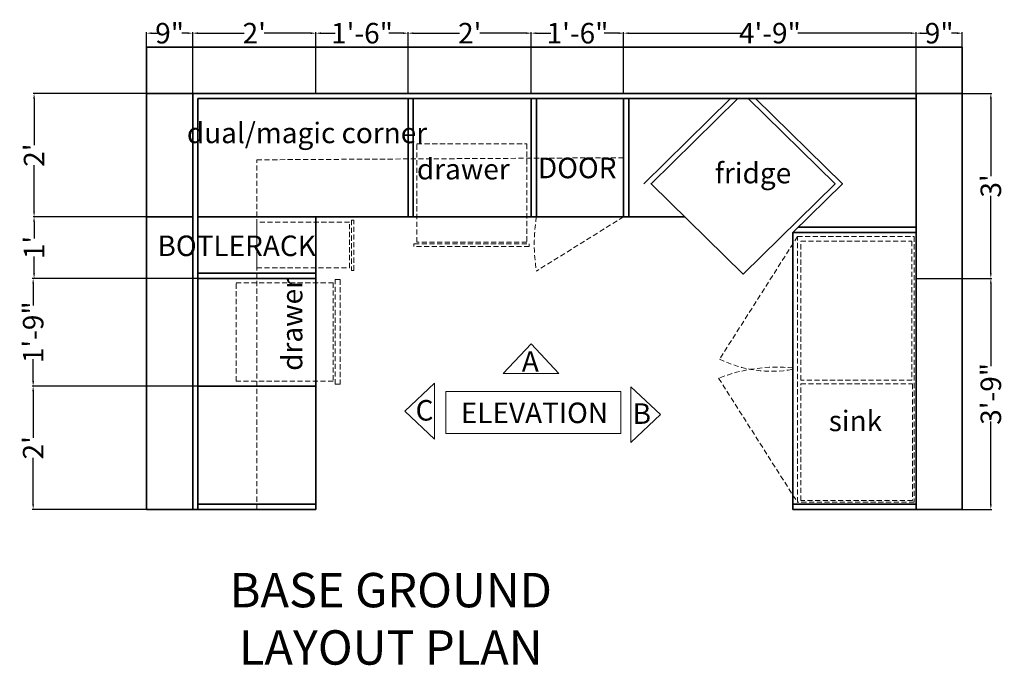
# Model space of a CAD drawing. Units: inches. Extents: x 560 to 756, y 301 to 635.
# Tile 2 of 2: x 564 to 756, y 509 to 635. Entities that reach past the tile are written whole.
import ezdxf

# ---------------------------------------------------------------- set-up
doc = ezdxf.new("R2010")
doc.units = ezdxf.units.IN
doc.header["$LTSCALE"] = 2
doc.header["$MEASUREMENT"] = 0
doc.linetypes.add('DASHED', pattern=[0.75, 0.5, -0.25])
for name, color, linetype, lineweight in [('A-ANNO-DIMS', 2, 'Continuous', 18), ('A-ANNO-SYMB', 7, 'Continuous', 18), ('A-ANNO-TEXT', 3, 'Continuous', 18), ('A-FURN', 7, 'Continuous', 35), ('A-FURN-OPEN', 8, 'DASHED', 18)]:
    doc.layers.add(name, color=color, linetype=linetype, lineweight=lineweight)
doc.styles.get("Standard").update_dxf_attribs({"font": 'arial.ttf'})
doc.dimstyles.get("Standard").update_dxf_attribs({"dimtxt": 4, "dimasz": 1, "dimexe": 0.18, "dimexo": 0.0625, "dimgap": 0.09, "dimtad": 0, "dimdec": 0, "dimzin": 0, "dimdsep": 46, "dimlunit": 4, "dimtxsty": 'Standard', "dimcen": 0.09, "dimadec": 0, "dimazin": 0, "dimtfac": 1, "dimtdec": 0, "dimtofl": 0, "dimtmove": 0, "dimatfit": 3, "dimfxl": 1, "dimtolj": 1, "dimtzin": 0, "dimarcsym": 0})

# ---------------------------------------------------------------- blocks, each defined once
blk = doc.blocks.new('*D1')
at = {"layer": 'A-ANNO-DIMS', "color": 0, "lineweight": -2, "transparency": 16777216}
for p, q in [((589.13, 620.48), (589.13, 632.34)), ((590.13, 632.16), (591.24, 632.16)), ((597.13, 632.16), (596.02, 632.16)), ((598.13, 620.48), (598.13, 632.34))]:
    blk.add_line(p, q, dxfattribs=at)
at = {"layer": 'A-ANNO-DIMS', "color": 0, "transparency": 16777216}
for points in [[(590.13, 632.33), (590.13, 632), (589.13, 632.16)], [(597.13, 632.33), (597.13, 632), (598.13, 632.16)]]:
    blk.add_solid(points, dxfattribs=at)
at = {"layer": 'Defpoints', "color": 0, "transparency": 16777216}
for p in [(598.13, 632.16), (589.13, 620.41), (598.13, 620.41)]:
    blk.add_point(p, dxfattribs=at)
at = {"layer": 'A-ANNO-DIMS', "color": 0, "transparency": 16777216, "insert": (593.63, 632.16), "char_height": 4, "attachment_point": 5}
blk.add_mtext('\\A1;9"', dxfattribs=at)
blk = doc.blocks.new('*D2')
at = {"layer": 'A-ANNO-DIMS', "color": 0, "lineweight": -2, "transparency": 16777216}
for p, q in [((598.13, 620.48), (598.13, 632.34)), ((599.13, 632.16), (608.16, 632.16)), ((621.13, 632.16), (612.09, 632.16)), ((622.13, 620.48), (622.13, 632.34))]:
    blk.add_line(p, q, dxfattribs=at)
at = {"layer": 'A-ANNO-DIMS', "color": 0, "transparency": 16777216}
for points in [[(599.13, 632.33), (599.13, 632), (598.13, 632.16)], [(621.13, 632.33), (621.13, 632), (622.13, 632.16)]]:
    blk.add_solid(points, dxfattribs=at)
at = {"layer": 'Defpoints', "color": 0, "transparency": 16777216}
for p in [(622.13, 632.16), (598.13, 620.41), (622.13, 620.41)]:
    blk.add_point(p, dxfattribs=at)
at = {"layer": 'A-ANNO-DIMS', "color": 0, "transparency": 16777216, "insert": (610.13, 632.16), "char_height": 4, "attachment_point": 5}
blk.add_mtext("\\A1;2'", dxfattribs=at)
blk = doc.blocks.new('*D3')
at = {"layer": 'A-ANNO-DIMS', "color": 0, "lineweight": -2, "transparency": 16777216}
for p, q in [((622.13, 620.48), (622.13, 632.34)), ((623.13, 632.16), (625.91, 632.16)), ((639.13, 632.16), (636.35, 632.16)), ((640.13, 620.48), (640.13, 632.34))]:
    blk.add_line(p, q, dxfattribs=at)
at = {"layer": 'A-ANNO-DIMS', "color": 0, "transparency": 16777216}
for points in [[(623.13, 632.33), (623.13, 632), (622.13, 632.16)], [(639.13, 632.33), (639.13, 632), (640.13, 632.16)]]:
    blk.add_solid(points, dxfattribs=at)
at = {"layer": 'Defpoints', "color": 0, "transparency": 16777216}
for p in [(640.13, 632.16), (622.13, 620.41), (640.13, 620.41)]:
    blk.add_point(p, dxfattribs=at)
at = {"layer": 'A-ANNO-DIMS', "color": 0, "transparency": 16777216, "insert": (631.13, 632.16), "char_height": 4, "attachment_point": 5}
blk.add_mtext('\\A1;1\'-6"', dxfattribs=at)
blk = doc.blocks.new('*D4')
at = {"layer": 'A-ANNO-DIMS', "color": 0, "lineweight": -2, "transparency": 16777216}
for p, q in [((640.13, 620.48), (640.13, 632.34)), ((641.13, 632.16), (650.16, 632.16)), ((663.13, 632.16), (654.09, 632.16)), ((664.13, 620.48), (664.13, 632.34))]:
    blk.add_line(p, q, dxfattribs=at)
at = {"layer": 'A-ANNO-DIMS', "color": 0, "transparency": 16777216}
for points in [[(641.13, 632.33), (641.13, 632), (640.13, 632.16)], [(663.13, 632.33), (663.13, 632), (664.13, 632.16)]]:
    blk.add_solid(points, dxfattribs=at)
at = {"layer": 'Defpoints', "color": 0, "transparency": 16777216}
for p in [(664.13, 632.16), (640.13, 620.41), (664.13, 620.41)]:
    blk.add_point(p, dxfattribs=at)
at = {"layer": 'A-ANNO-DIMS', "color": 0, "transparency": 16777216, "insert": (652.13, 632.16), "char_height": 4, "attachment_point": 5}
blk.add_mtext("\\A1;2'", dxfattribs=at)
blk = doc.blocks.new('*D5')
at = {"layer": 'A-ANNO-DIMS', "color": 0, "lineweight": -2, "transparency": 16777216}
for p, q in [((664.13, 620.48), (664.13, 632.34)), ((665.13, 632.16), (667.91, 632.16)), ((681.13, 632.16), (678.35, 632.16)), ((682.13, 620.48), (682.13, 632.34))]:
    blk.add_line(p, q, dxfattribs=at)
at = {"layer": 'A-ANNO-DIMS', "color": 0, "transparency": 16777216}
for points in [[(665.13, 632.33), (665.13, 632), (664.13, 632.16)], [(681.13, 632.33), (681.13, 632), (682.13, 632.16)]]:
    blk.add_solid(points, dxfattribs=at)
at = {"layer": 'Defpoints', "color": 0, "transparency": 16777216}
for p in [(682.13, 632.16), (664.13, 620.41), (682.13, 620.41)]:
    blk.add_point(p, dxfattribs=at)
at = {"layer": 'A-ANNO-DIMS', "color": 0, "transparency": 16777216, "insert": (673.13, 632.16), "char_height": 4, "attachment_point": 5}
blk.add_mtext('\\A1;1\'-6"', dxfattribs=at)
blk = doc.blocks.new('*D6')
at = {"layer": 'A-ANNO-DIMS', "color": 0, "lineweight": -2, "transparency": 16777216}
for p, q in [((682.13, 620.48), (682.13, 632.34)), ((683.13, 632.16), (705.14, 632.16)), ((738.13, 632.16), (716.11, 632.16)), ((739.13, 620.48), (739.13, 632.34))]:
    blk.add_line(p, q, dxfattribs=at)
at = {"layer": 'A-ANNO-DIMS', "color": 0, "transparency": 16777216}
for points in [[(683.13, 632.33), (683.13, 632), (682.13, 632.16)], [(738.13, 632.33), (738.13, 632), (739.13, 632.16)]]:
    blk.add_solid(points, dxfattribs=at)
at = {"layer": 'Defpoints', "color": 0, "transparency": 16777216}
for p in [(739.13, 632.16), (682.13, 620.41), (739.13, 620.41)]:
    blk.add_point(p, dxfattribs=at)
at = {"layer": 'A-ANNO-DIMS', "color": 0, "transparency": 16777216, "insert": (710.63, 632.16), "char_height": 4, "attachment_point": 5}
blk.add_mtext('\\A1;4\'-9"', dxfattribs=at)
blk = doc.blocks.new('*D7')
at = {"layer": 'A-ANNO-DIMS', "color": 0, "lineweight": -2, "transparency": 16777216}
for p, q in [((739.13, 620.48), (739.13, 632.34)), ((740.13, 632.16), (741.24, 632.16)), ((747.13, 632.16), (746.02, 632.16)), ((748.13, 620.48), (748.13, 632.34))]:
    blk.add_line(p, q, dxfattribs=at)
at = {"layer": 'A-ANNO-DIMS', "color": 0, "transparency": 16777216}
for points in [[(740.13, 632.33), (740.13, 632), (739.13, 632.16)], [(747.13, 632.33), (747.13, 632), (748.13, 632.16)]]:
    blk.add_solid(points, dxfattribs=at)
at = {"layer": 'Defpoints', "color": 0, "transparency": 16777216}
for p in [(739.13, 632.16), (739.13, 620.41), (748.13, 620.41)]:
    blk.add_point(p, dxfattribs=at)
at = {"layer": 'A-ANNO-DIMS', "color": 0, "transparency": 16777216, "insert": (743.63, 632.16), "char_height": 4, "attachment_point": 5}
blk.add_mtext('\\A1;9"', dxfattribs=at)
blk = doc.blocks.new('*D8')
at = {"layer": 'A-ANNO-DIMS', "color": 0, "lineweight": -2, "transparency": 16777216}
for p, q in [((589.06, 620.41), (567.03, 620.41)), ((567.21, 619.41), (567.21, 610.38)), ((567.21, 597.41), (567.21, 606.45)), ((589.06, 596.41), (567.03, 596.41))]:
    blk.add_line(p, q, dxfattribs=at)
at = {"layer": 'A-ANNO-DIMS', "color": 0, "transparency": 16777216}
for points in [[(567.04, 619.41), (567.38, 619.41), (567.21, 620.41)], [(567.04, 597.41), (567.38, 597.41), (567.21, 596.41)]]:
    blk.add_solid(points, dxfattribs=at)
at = {"layer": 'Defpoints', "color": 0, "transparency": 16777216}
for p in [(589.13, 620.41), (567.21, 596.41), (589.13, 596.41)]:
    blk.add_point(p, dxfattribs=at)
at = {"layer": 'A-ANNO-DIMS', "color": 0, "transparency": 16777216, "insert": (567.21, 608.41), "char_height": 4, "attachment_point": 5, "rotation": 90}
blk.add_mtext("\\A1;2'", dxfattribs=at)
blk = doc.blocks.new('*D9')
at = {"layer": 'A-ANNO-DIMS', "color": 0, "lineweight": -2, "transparency": 16777216}
for p, q in [((598.06, 596.41), (567.03, 596.41)), ((567.21, 595.41), (567.21, 592.16)), ((567.21, 585.41), (567.21, 588.67)), ((598.06, 584.41), (567.03, 584.41))]:
    blk.add_line(p, q, dxfattribs=at)
at = {"layer": 'A-ANNO-DIMS', "color": 0, "transparency": 16777216}
for points in [[(567.04, 595.41), (567.38, 595.41), (567.21, 596.41)], [(567.04, 585.41), (567.38, 585.41), (567.21, 584.41)]]:
    blk.add_solid(points, dxfattribs=at)
at = {"layer": 'Defpoints', "color": 0, "transparency": 16777216}
for p in [(598.13, 596.41), (567.21, 584.41), (598.13, 584.41)]:
    blk.add_point(p, dxfattribs=at)
at = {"layer": 'A-ANNO-DIMS', "color": 0, "transparency": 16777216, "insert": (567.21, 590.41), "char_height": 4, "attachment_point": 5, "rotation": 90}
blk.add_mtext("\\A1;1'", dxfattribs=at)
blk = doc.blocks.new('*D10')
at = {"layer": 'A-ANNO-DIMS', "color": 0, "lineweight": -2, "transparency": 16777216}
for p, q in [((739.19, 620.41), (753.88, 620.41)), ((753.7, 619.41), (753.7, 604.34)), ((753.7, 585.41), (753.7, 600.49)), ((739.19, 584.41), (753.88, 584.41))]:
    blk.add_line(p, q, dxfattribs=at)
at = {"layer": 'A-ANNO-DIMS', "color": 0, "transparency": 16777216}
for points in [[(753.53, 619.41), (753.87, 619.41), (753.7, 620.41)], [(753.53, 585.41), (753.87, 585.41), (753.7, 584.41)]]:
    blk.add_solid(points, dxfattribs=at)
at = {"layer": 'Defpoints', "color": 0, "transparency": 16777216}
for p in [(739.13, 620.41), (739.13, 584.41), (753.7, 584.41)]:
    blk.add_point(p, dxfattribs=at)
at = {"layer": 'A-ANNO-DIMS', "color": 0, "transparency": 16777216, "insert": (753.7, 602.41), "char_height": 4, "attachment_point": 5, "rotation": 90}
blk.add_mtext("\\A1;3'", dxfattribs=at)
blk = doc.blocks.new('*D11')
at = {"layer": 'A-ANNO-DIMS', "color": 0, "lineweight": -2, "transparency": 16777216}
for p, q in [((739.19, 584.41), (753.88, 584.41)), ((753.7, 583.41), (753.7, 567.32)), ((753.7, 540.41), (753.7, 556.51)), ((739.19, 539.41), (753.88, 539.41))]:
    blk.add_line(p, q, dxfattribs=at)
at = {"layer": 'A-ANNO-DIMS', "color": 0, "transparency": 16777216}
for points in [[(753.53, 583.41), (753.87, 583.41), (753.7, 584.41)], [(753.53, 540.41), (753.87, 540.41), (753.7, 539.41)]]:
    blk.add_solid(points, dxfattribs=at)
at = {"layer": 'Defpoints', "color": 0, "transparency": 16777216}
for p in [(739.13, 584.41), (739.13, 539.41), (753.7, 539.41)]:
    blk.add_point(p, dxfattribs=at)
at = {"layer": 'A-ANNO-DIMS', "color": 0, "transparency": 16777216, "insert": (753.7, 561.91), "char_height": 4, "attachment_point": 5, "rotation": 90}
blk.add_mtext('\\A1;3\'-9"', dxfattribs=at)
blk = doc.blocks.new('*D12')
at = {"layer": 'A-ANNO-DIMS', "color": 0, "lineweight": -2, "transparency": 16777216}
for p, q in [((599.06, 584.41), (566.85, 584.41)), ((567.03, 583.41), (567.03, 579.13)), ((567.03, 564.41), (567.03, 568.7)), ((599.06, 563.41), (566.85, 563.41))]:
    blk.add_line(p, q, dxfattribs=at)
at = {"layer": 'A-ANNO-DIMS', "color": 0, "transparency": 16777216}
for points in [[(566.86, 583.41), (567.2, 583.41), (567.03, 584.41)], [(566.86, 564.41), (567.2, 564.41), (567.03, 563.41)]]:
    blk.add_solid(points, dxfattribs=at)
at = {"layer": 'Defpoints', "color": 0, "transparency": 16777216}
for p in [(599.13, 584.41), (567.03, 563.41), (599.13, 563.41)]:
    blk.add_point(p, dxfattribs=at)
at = {"layer": 'A-ANNO-DIMS', "color": 0, "transparency": 16777216, "insert": (567.03, 573.91), "char_height": 4, "attachment_point": 5, "rotation": 90}
blk.add_mtext('\\A1;1\'-9"', dxfattribs=at)
blk = doc.blocks.new('*D13')
at = {"layer": 'A-ANNO-DIMS', "color": 0, "lineweight": -2, "transparency": 16777216}
for p, q in [((589.06, 563.41), (566.85, 563.41)), ((567.03, 562.41), (567.03, 553.38)), ((567.03, 540.41), (567.03, 549.45)), ((589.06, 539.41), (566.85, 539.41))]:
    blk.add_line(p, q, dxfattribs=at)
at = {"layer": 'A-ANNO-DIMS', "color": 0, "transparency": 16777216}
for points in [[(566.86, 562.41), (567.2, 562.41), (567.03, 563.41)], [(566.86, 540.41), (567.2, 540.41), (567.03, 539.41)]]:
    blk.add_solid(points, dxfattribs=at)
at = {"layer": 'Defpoints', "color": 0, "transparency": 16777216}
for p in [(589.13, 563.41), (567.03, 539.41), (589.13, 539.41)]:
    blk.add_point(p, dxfattribs=at)
at = {"layer": 'A-ANNO-DIMS', "color": 0, "transparency": 16777216, "insert": (567.03, 551.41), "char_height": 4, "attachment_point": 5, "rotation": 90}
blk.add_mtext("\\A1;2'", dxfattribs=at)

msp = doc.modelspace()

# ---------------------------------------------------------------- linework, layer by layer
at = {"layer": 'A-ANNO-SYMB'}
for points in [[(658.64, 565.87), (669.52, 565.87), (664.08, 571.67)], [(645.28, 553.1), (645.28, 563.98), (639.48, 558.54)], [(647.49, 562.36), (681.56, 562.36), (681.56, 554.18), (647.49, 554.18)], [(683.51, 552.43), (683.51, 563.31), (689.31, 557.87)]]:
    msp.add_lwpolyline(points, close=True, dxfattribs=at)
at = {"layer": 'A-FURN'}
for p, q in [((589.13, 620.41), (589.13, 629.41)), ((589.13, 629.41), (748.13, 629.41)), ((748.13, 620.41), (748.13, 629.41)), ((589.13, 620.41), (598.13, 620.41)), ((589.13, 620.41), (589.13, 596.41)), ((739.13, 620.41), (748.13, 620.41)), ((739.13, 620.41), (739.13, 584.41)), ((748.13, 539.41), (748.13, 620.41)), ((640.13, 619.41), (640.13, 596.41)), ((641.13, 619.41), (641.13, 596.41)), ((664.13, 619.41), (664.13, 596.41)), ((665.13, 619.41), (665.13, 596.41)), ((682.13, 619.41), (682.13, 596.41)), ((683.13, 619.41), (683.13, 596.41)), ((589.13, 596.41), (589.13, 584.41)), ((589.13, 596.41), (598.13, 596.41)), ((599.13, 596.41), (640.13, 596.41)), ((622.13, 539.41), (622.13, 596.41)), ((640.13, 596.41), (664.13, 596.41)), ((664.13, 596.41), (682.13, 596.41)), ((682.13, 596.41), (694, 596.41)), ((715.13, 593.37), (715.13, 584.41)), ((715.13, 593.37), (739.13, 593.37)), ((716.15, 594.37), (739.13, 594.37)), ((599.13, 585.41), (622.13, 585.41)), ((589.13, 584.41), (589.13, 563.41)), ((599.13, 584.41), (622.13, 584.41)), ((715.13, 584.41), (715.13, 539.41)), ((739.13, 584.41), (739.13, 539.41)), ((589.13, 563.41), (589.13, 539.41)), ((599.13, 563.41), (622.13, 563.41)), ((589.13, 539.41), (622.13, 539.41)), ((599.13, 540.41), (622.13, 540.41)), ((715.13, 540.41), (739.13, 540.41)), ((715.13, 539.41), (748.13, 539.41))]:
    msp.add_line(p, q, dxfattribs=at)
for points in [[(598.13, 539.41), (598.13, 620.41), (622.13, 620.41), (640.13, 620.41), (664.13, 620.41), (682.13, 620.41), (739.13, 620.41)], [(599.13, 539.41), (599.13, 619.41), (622.13, 619.41), (640.13, 619.41), (664.13, 619.41), (682.13, 619.41), (739.13, 619.41)], [(702.95, 619.41), (686.04, 602.82)], [(704.38, 619.41), (687.47, 602.82), (705.4, 585.23), (723.33, 602.82), (706.42, 619.41)], [(715.13, 593.37), (724.76, 602.82), (707.85, 619.41)]]:
    msp.add_lwpolyline(points, dxfattribs=at)
at = {"layer": 'A-FURN-OPEN'}
for p, q in [((610.63, 607.5), (682.13, 607.91)), ((610.63, 539.41), (610.63, 607.5)), ((682.13, 596.41), (665.13, 585.83)), ((716.01, 592.54), (700.82, 568.67)), ((700.64, 564.96), (716.01, 540.8))]:
    msp.add_line(p, q, dxfattribs=at)
for points in [[(641.82, 610.6), (663.28, 610.6), (663.28, 591.45), (641.82, 591.45)], [(610.63, 586.46), (628.69, 586.46), (628.69, 595.35), (610.63, 595.35)], [(629.05, 585.96), (629.54, 585.96), (629.54, 595.75), (629.05, 595.75)], [(641.26, 591.14), (663.73, 591.14), (663.73, 590.63), (641.26, 590.63)], [(716.01, 592.54), (738.76, 592.54), (738.76, 540.8), (716.01, 540.8)], [(716.65, 591.68), (738.33, 591.68), (738.33, 564.56), (716.65, 564.56)], [(606.57, 583.56), (625.53, 583.56), (625.53, 564.39), (606.57, 564.39)], [(625.87, 584.18), (626.84, 584.18), (626.84, 563.77), (625.87, 563.77)], [(716.64, 563.84), (738.44, 563.84), (738.44, 541.13), (716.64, 541.13)]]:
    msp.add_lwpolyline(points, close=True, dxfattribs=at)
for centre, radius, start, end in [((698.29, 591.12), 33.58, 170.933, 189.067), ((711.02, 589.52), 23.21, 243.9058, 280.1835), ((711.94, 536.51), 30.61, 84.0322, 111.6808)]:
    msp.add_arc(centre, radius, start, end, dxfattribs=at)

# ---------------------------------------------------------------- texts
at = {"layer": 'A-ANNO-TEXT'}
for s, width, gutter_width, insert, char_height, attachment_point in [('dual/magic corner', 48.4721, 20, (596.98, 614.74), 4, 1), ('drawer', 21.4632, 20, (641.82, 607.68), 4, 1), ('DOOR', 16.7117, 20, (665.42, 607.91), 4, 1), ('\\pxqc;fridge', 21.761, 20, (696.47, 606.91), 4, 1), ('BOTLERACK', 34.2246, 20, (591.26, 592.75), 4, 1), ('A', 8.9657, 20, (662.28, 570.22), 4, 1), ('C', 8.9657, 20, (641.57, 560.71), 4, 1), ('\\pxqc;ELEVATION', 26.9266, 20, (651.28, 560.21), 4, 1), ('B', 8.9657, 20, (683.88, 556.07), 4, 7), ('\\pxqc;sink', 17.7642, 20, (718.43, 558.65), 4, 1), ('\\pxqc;BASE GROUND\\PLAYOUT PLAN', 203.4879, 33.51, (535, 527.04), 6.7011, 1)]:
    msp.add_mtext_dynamic_manual_height_columns(s, width=width, gutter_width=gutter_width, heights=[0], dxfattribs=dict(at, insert=insert, char_height=char_height, attachment_point=attachment_point))
at = {"layer": 'A-ANNO-TEXT', "insert": (615.5, 566.39), "char_height": 4, "attachment_point": 1, "rotation": 90}
msp.add_mtext_dynamic_manual_height_columns('drawer', width=21.4632, gutter_width=20, heights=[0], dxfattribs=at)

# ---------------------------------------------------------------- dimensions: what is measured, and where the dimension line sits
at = {"layer": 'A-ANNO-DIMS'}
for base, p1, p2, picture, middle in [((598.13, 632.16), (589.13, 620.41), (598.13, 620.41), '*D1', (593.63, 632.16)), ((622.13, 632.16), (598.13, 620.41), (622.13, 620.41), '*D2', (610.13, 632.16)), ((640.13, 632.16), (622.13, 620.41), (640.13, 620.41), '*D3', (631.13, 632.16)), ((664.13, 632.16), (640.13, 620.41), (664.13, 620.41), '*D4', (652.13, 632.16)), ((682.13, 632.16), (664.13, 620.41), (682.13, 620.41), '*D5', (673.13, 632.16)), ((739.13, 632.16), (682.13, 620.41), (739.13, 620.41), '*D6', (710.63, 632.16)), ((739.13, 632.16), (748.13, 620.41), (739.13, 620.41), '*D7', (743.63, 632.16))]:
    dim = msp.add_linear_dim(base=base, p1=p1, p2=p2, dimstyle='Standard', override={"dimclrd": 0, "dimclre": 0, "dimclrt": 0}, dxfattribs=at)
    dim.commit()
    dim.dimension.update_dxf_attribs({"geometry": picture, "text_midpoint": middle})
for base, p1, p2, picture, middle in [((567.21, 596.41), (589.13, 620.41), (589.13, 596.41), '*D8', (567.21, 608.41)), ((753.7, 584.41), (739.13, 620.41), (739.13, 584.41), '*D10', (753.7, 602.41)), ((567.21, 584.41), (598.13, 596.41), (598.13, 584.41), '*D9', (567.21, 590.41)), ((567.03, 563.41), (599.13, 584.41), (599.13, 563.41), '*D12', (567.03, 573.91)), ((753.7, 539.41), (739.13, 584.41), (739.13, 539.41), '*D11', (753.7, 561.91)), ((567.03, 539.41), (589.13, 563.41), (589.13, 539.41), '*D13', (567.03, 551.41))]:
    dim = msp.add_linear_dim(base=base, p1=p1, p2=p2, angle=90, dimstyle='Standard', override={"dimclrd": 0, "dimclre": 0, "dimclrt": 0}, dxfattribs=at)
    dim.commit()
    dim.dimension.update_dxf_attribs({"geometry": picture, "text_midpoint": middle})

doc.saveas('drawing.dxf')
